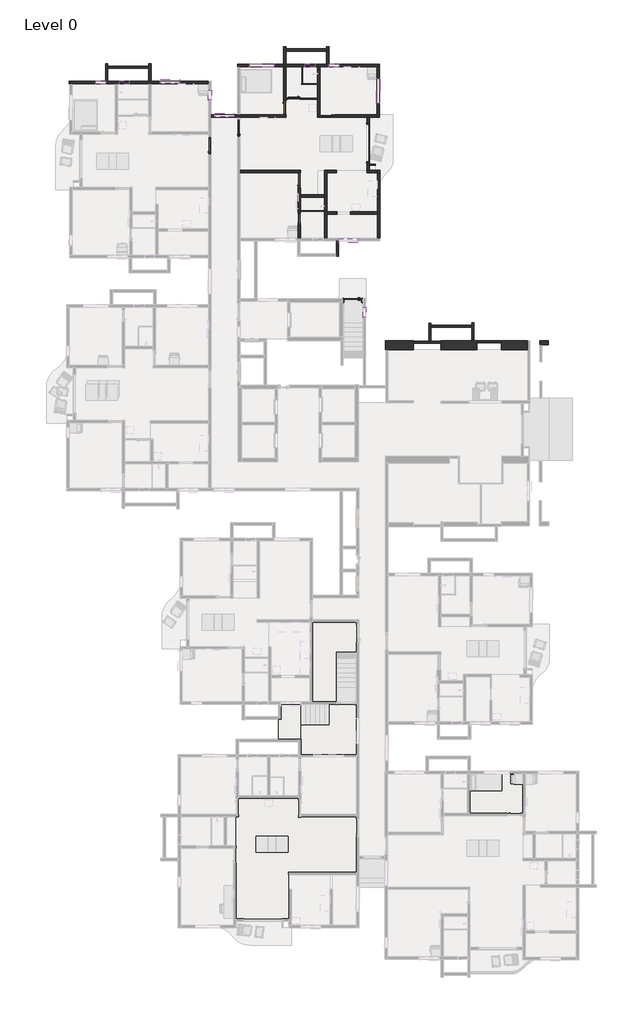
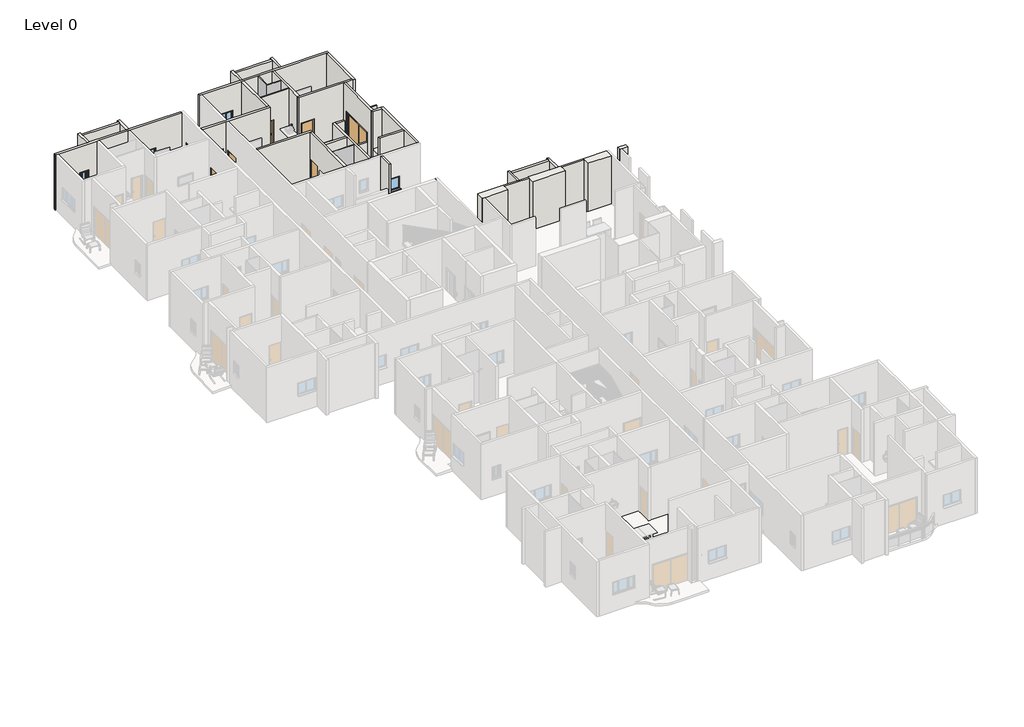
# One storey, part 7 of 14: 35 walls, 11 windows, 9 doors, 5 slabs, 3 plates.
# Revit data of these elements (continued)
# Type "Windows_Tpl_Variable_Casement : 2'" (continued)
#   Wrap Layers (Int) from Ext = 177.5 mm
#   Wrap Layers (Ext) from Ext = 102.5 mm
#   Window Board Projection = 25 mm
#   Window Board Extension = 25 mm
#   Visual Light Transmittance = 0.9
#   Solar Heat Gain Coefficient = 0.78
#   Rough Width = 609.6 mm
#   Rough Height = 910 mm
#   Height = 910 mm
#   Width = 609.6 mm
#   Heat Transfer Coefficient (U) = 3.6886 W/(m²·K)
#   Glazing Thickness = 24 mm
#   FrameOffset - External = 50 mm
#   Frame Depth = 65 mm
#   Default Head Height = 2110 mm
#   Cill Depth = 87.5 mm
#   Cavity Closer Width = 50 mm
#   Cavity Closer Offset from Ext = 102.5 mm
#   Cavity Closer Depth = 85 mm
#   Casement Width = 450 mm
#   Vis - Cavity Closers = yes
#   Define Thermal Properties by = 1
#   Material Trim = Window Frame
#   Material Glass = Glass
#   Material Frame = Window Frame
#   Wall Closure = (empty or 0)
# Type "Windows_Tpl_Variable_Casement : 5'"
#   Type Mark = "83"
#   Operation = "TriplePanelVertical"
#   Construction Type Id = "GSP4R"
#   Manufacturer = "Revit"
#   Keynote = "L10"
#   Analytic Construction = "1/8 in Pilkington single glazing"
#   Wrap Layers (Int) from Ext = 177.5 mm
#   Wrap Layers (Ext) from Ext = 102.5 mm
#   Window Board Projection = 25 mm
#   Window Board Extension = 25 mm
#   Visual Light Transmittance = 0.9
#   Solar Heat Gain Coefficient = 0.78
#   Rough Width = 1524 mm
#   Rough Height = 910 mm
#   Height = 910 mm
#   Width = 1524 mm
#   Heat Transfer Coefficient (U) = 3.6886 W/(m²·K)
#   Glazing Thickness = 24 mm
#   FrameOffset - External = 50 mm
#   Frame Depth = 65 mm
#   Default Head Height = 2110 mm
#   Cill Depth = 87.5 mm
#   Cavity Closer Width = 50 mm
#   Cavity Closer Offset from Ext = 102.5 mm
#   Cavity Closer Depth = 85 mm
#   Casement Width = 450 mm
#   Vis - Cavity Closers = yes
#   Define Thermal Properties by = 1
#   Material Trim = Window Frame
#   Material Glass = Glass
#   Material Frame = Window Frame
#   Wall Closure = (empty or 0)
# Element 1 (IfcDoor, "Doors_Concept_IntDbl : 8'")
#   Phase Created = New Construction
#   Materials on its faces: "Glass", "Glass, Clear Glazing"
# Elements 2, 3 (IfcDoor, "Doors_ExtSgl_Flush : D1")
#   Phase Created = New Construction
#   Materials on its faces: "Door - Handle", "Door - Frame/Mullion", "Door - Panel"
# Elements 4, 5, 6 (IfcDoor, "Doors_ExtSgl_Flush : D2")
#   Phase Created = New Construction
#   Materials on its faces: "Door - Handle", "Door - Frame/Mullion", "Door - Panel"
# Elements 7, 8 (IfcDoor, "Doors_ExtSgl_Flush : D3")
#   Phase Created = New Construction
#   Materials on its faces: "Door - Handle", "Door - Frame/Mullion", "Door - Panel"
# Element 9 (IfcDoor, "Doors_IntSgl : 3.75'")
#   Phase Created = New Construction
#   Materials on its faces: "Door - Architrave", "Door - Handle", "Door - Frame/Mullion (1)", "Door - Panel"
# Elements 10, 11, 12 (IfcPlate, "System Panel : Glazed")
#   Phase Created = New Construction
#   Materials on its faces: "Glass"
# Element 13 (IfcSlab)
#   Height Offset From Level = 149.962 mm
#   Phase Created = New Construction
#   Materials on its faces: "Structure, Timber Joist/Rafter Layer", "KITCHEN"
# Element 14 (IfcSlab, "OUTDOOR")
#   built-in parameter 1001955 = 1.5708 (stored number, unit not read)
#   Height Offset From Level = 1000 mm
#   Phase Created = New Construction
#   Materials on its faces: "Structure, Timber Joist/Rafter Layer", "OUTDOOR FLOORING"
# Element 15 (IfcSlab, "OUTDOOR")
#   built-in parameter 1001955 = 3.14159 (stored number, unit not read)
#   Height Offset From Level = 149.962 mm
#   Phase Created = New Construction
#   Materials on its faces: "Structure, Timber Joist/Rafter Layer", "OUTDOOR FLOORING"
# Element 16 (IfcSlab, "STAIRCASE FLOORING")
#   Height Offset From Level = 149.962 mm
#   Phase Created = New Construction
#   Materials on its faces: "Structure, Timber Joist/Rafter Layer", "Wood Sheathing, Chipboard"
# Element 17 (IfcSlab, "STUDY ROOM")
#   Height Offset From Level = 149.962 mm
#   Phase Created = New Construction
#   Materials on its faces: "Structure, Timber Joist/Rafter Layer", "KITCHEN"
# Elements 18, 19, 20, 21, 22, 23, 24, 25, 26, 27, 28, 29, 30, 31, 32, 33, 34, 35, 36, 37, 38, 39, 40, 41 (IfcWall, "W1")
#   Top Offset = 0 mm
#   Base Offset = 0 mm
#   wall height = 4000 mm
#   Phase Created = New Construction
#   Base Constraint = Level 0
#   Top Constraint = Level 1
#   Materials on its faces: "Brick, Common"
# Elements 42, 43 (IfcWall, "W2")
#   Top Offset = 0 mm
#   Base Offset = 0 mm
#   wall height = 4000 mm
#   Phase Created = New Construction
#   Base Constraint = Level 0
#   Top Constraint = Level 1
#   Materials on its faces: "Brick, Common"
# Element 44 (IfcWall, "W3")
#   Top Offset = 0 mm
#   Base Offset = 0 mm
#   wall height = 4000 mm
#   Phase Created = New Construction
#   Base Constraint = Level 0
#   Top Constraint = Level 1
#   Materials on its faces: "Brick, Common"
# Elements 45, 46, 47, 48, 49 (IfcWall, "W6")
#   Top Offset = 0 mm
#   Base Offset = 0 mm
#   wall height = 4000 mm
#   Phase Created = New Construction
#   Base Constraint = Level 0
#   Top Constraint = Level 1
#   Materials on its faces: "Brick, Common"
# Elements 50, 51, 52 (IfcWall, "W7")
#   Top Offset = 0 mm
#   Base Offset = 0 mm
#   wall height = 4000 mm
#   Phase Created = New Construction
#   Base Constraint = Level 0
#   Top Constraint = Level 1
#   Materials on its faces: "Brick, Common"
# Element 53 (IfcWindow, "Windows_Concept_Plain_Dbl : 4'")
#   Mark = "35"
#   Phase Created = New Construction
#   Materials on its faces: "Window Frame", "Glass"
# Element 54 (IfcWindow, "Windows_Concept_Plain_Dbl : 4'")
#   Mark = "43"
#   Phase Created = New Construction
#   Materials on its faces: "Window Frame", "Glass"
# Element 55 (IfcWindow, "Windows_Concept_Plain_Dbl : 4'")
#   Mark = "72"
#   Phase Created = New Construction
#   Materials on its faces: "Window Frame", "Glass"
# Element 56 (IfcWindow, "Windows_Sgl_Plain : 2'")
#   Mark = "41"
#   Phase Created = New Construction
#   Materials on its faces: "Window Frame", "Glass"
# Element 57 (IfcWindow, "Windows_Sgl_Plain : 2'")
#   Mark = "49"
#   Phase Created = New Construction
#   Materials on its faces: "Window Frame", "Glass"
# Element 58 (IfcWindow, "Windows_Tpl_Variable_Casement : 2'")
#   Mark = "38"
#   Phase Created = New Construction
#   Materials on its faces: "Window Frame", "Glass"
# Element 59 (IfcWindow, "Windows_Tpl_Variable_Casement : 2'")
#   Mark = "42"
#   Phase Created = New Construction
#   Materials on its faces: "Window Frame", "Glass"
# Element 60 (IfcWindow, "Windows_Tpl_Variable_Casement : 2'")
#   Mark = "44"
#   Phase Created = New Construction
#   Materials on its faces: "Window Frame", "Glass"
# Element 61 (IfcWindow, "Windows_Tpl_Variable_Casement : 2'")
#   Mark = "33"
#   Phase Created = New Construction
#   Materials on its faces: "Window Frame", "Glass"
# Element 62 (IfcWindow, "Windows_Tpl_Variable_Casement : 5'")
#   Mark = "37"
#   Phase Created = New Construction
#   Materials on its faces: "Window Frame", "Glass"
# Element 63 (IfcWindow, "Windows_Tpl_Variable_Casement : 5'")
#   Mark = "39"
#   Phase Created = New Construction
#   Materials on its faces: "Window Frame", "Glass"
# Materials
#   "Glass": class "Glass", colour RGB 0 128 192, transparency 0.9, Description = "Soda Lime Glass", Cost = 0
#   "Glass, Clear Glazing": class "Glass", colour RGB 0 128 192, transparency 0.75, Description = "Clear glazing", Cost = 0
#   "Door - Panel": class "Wood", colour RGB 210 159 95, transparency 0, Keynote = "L20", Cost = 0
#   "Door - Frame/Mullion": class "Wood", colour RGB 212 179 113, transparency 0, Keynote = "L20", Cost = 0
#   "Door - Handle": colour RGB 0 0 0, transparency 0, Keynote = "P21", Cost = 0
#   "Door - Frame/Mullion (1)": class "Wood", colour RGB 212 179 113, transparency 0, Keynote = "L20", Cost = 0
#   "Door - Architrave": class "Wood", colour RGB 154 90 5, transparency 0, Keynote = "P20", Cost = 0
#   "KITCHEN": class "Generic", colour RGB 120 120 120, transparency 0, Cost = 0
#   "Structure, Timber Joist/Rafter Layer": class "Wood", colour RGB 127 127 127, transparency 0, Description = "Timber framing, thermal airspace", Cost = 0
#   "OUTDOOR FLOORING": class "Generic", colour RGB 120 120 120, transparency 0, Cost = 0
#   "Wood Sheathing, Chipboard": class "Wood", colour RGB 127 127 127, transparency 0, Description = "Particleboard sheathing", Cost = 0
#   "Brick, Common": class "Masonry", colour RGB 170 100 105, transparency 0, Description = "Common brick", Cost = 0
#   "Window Frame": colour RGB 249 249 249, transparency 0, Keynote = "L10", Cost = 0
